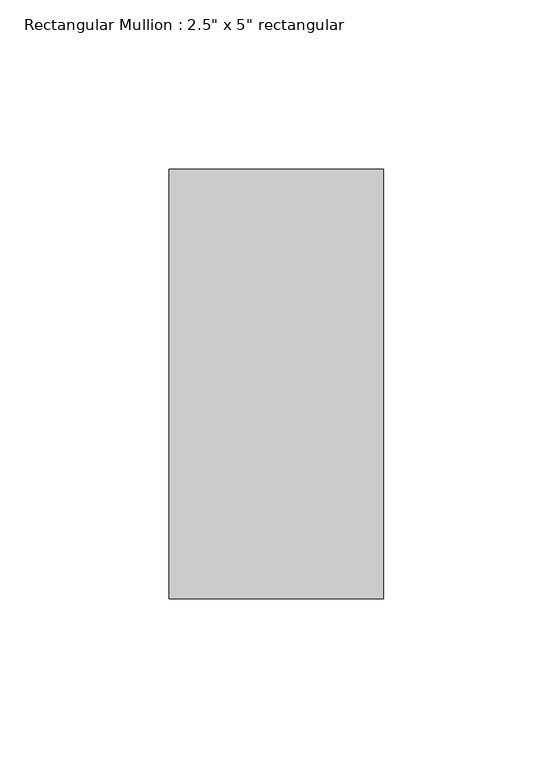
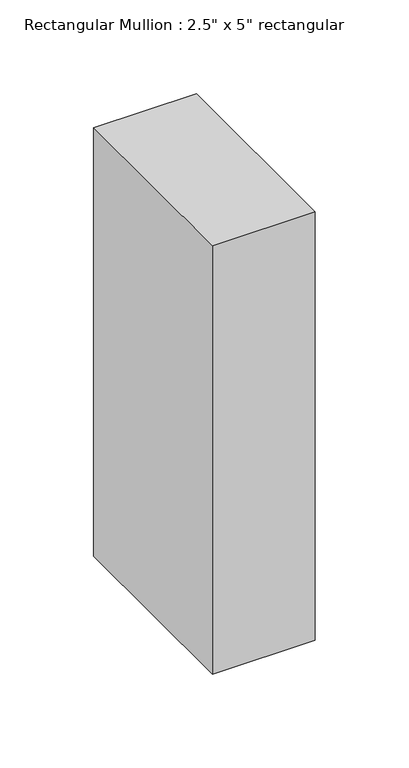
"""IFC4 building model written with IfcOpenShell, lengths in millimetres: member geometry."""

from ifc_helpers import new_model, si_unit, frame, origin, place, context, project, spatial, polyline, outline, extrude, source, transform, mapped, element, save


def member_d3323a85(model_context):
    return source(origin(), model_context, "Body", "SweptSolid", [
        extrude(outline(polyline([(0.0, 63.5), (0.0, -63.5), (-63.5, -63.5), (-63.5, 63.5), (0.0, 63.5)])), frame((0.0, 0.0, -279.4), z_axis=(0.0, 0.0, 1.0), x_axis=(1.0, 0.0, 0.0)), (0.0, 0.0, 1.0), 279.4),
    ])


if __name__ == "__main__":
    model = new_model("IFC4")
    model_context = context("Model", 3, world=origin())
    ifc_project = project(units=[si_unit("LENGTHUNIT", "METRE", prefix="MILLI")], contexts=[model_context])
    site = spatial("IfcSite", under=ifc_project)
    building = spatial("IfcBuilding", under=site)
    placement = place(None, origin())
    member_shape = member_d3323a85(model_context)
    element("IfcMember", 1, ObjectType="Rectangular Mullion : 2.5\" x 5\" rectangular", at=placement, inside=building, context=model_context, shape_type="MappedRepresentation", body=[
        mapped(member_shape, transform((0.0, 0.0, 0.0), x_axis=(1.0, 0.0, 0.0), y_axis=(0.0, 1.0, 0.0), z_axis=(0.0, 0.0, 1.0))),
    ])
    save(model, "model.ifc")

# Revit data of these elements
# Type "Rectangular Mullion : 2.5\" x 5\" rectangular"
#   built-in parameter 1007304 = 0.416667 (stored number, unit not read)
#   built-in parameter 1007301 = 0.104167 (stored number, unit not read)
#   built-in parameter 1007300 = 0.104167 (stored number, unit not read)
